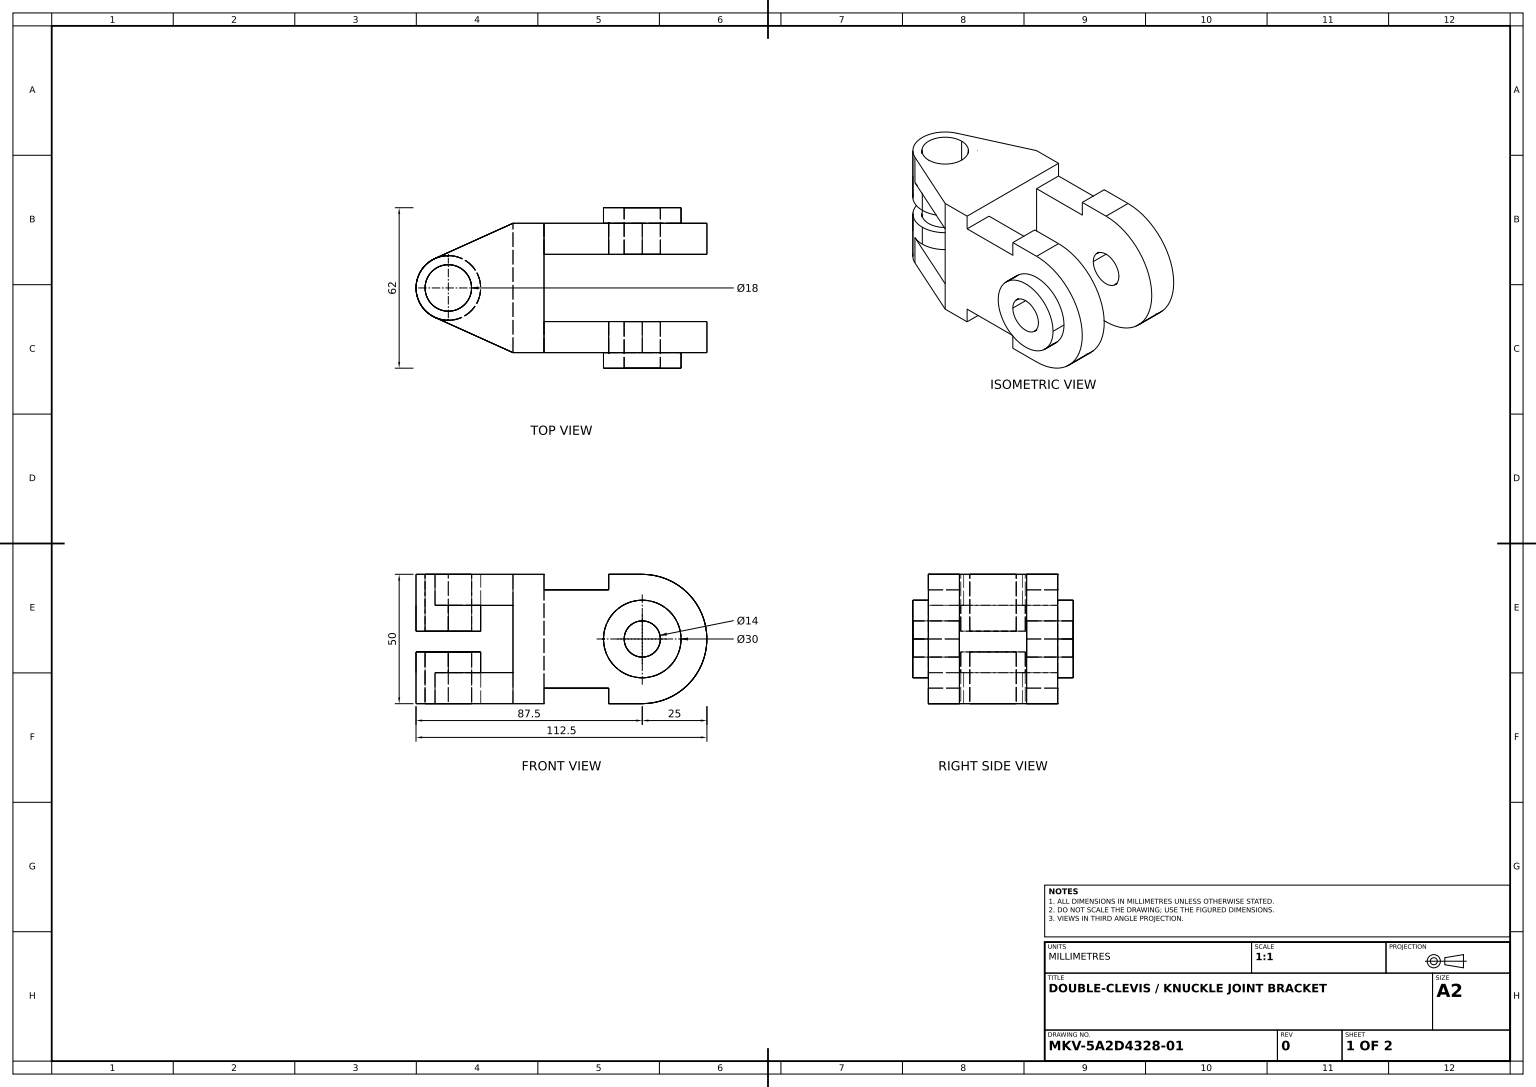
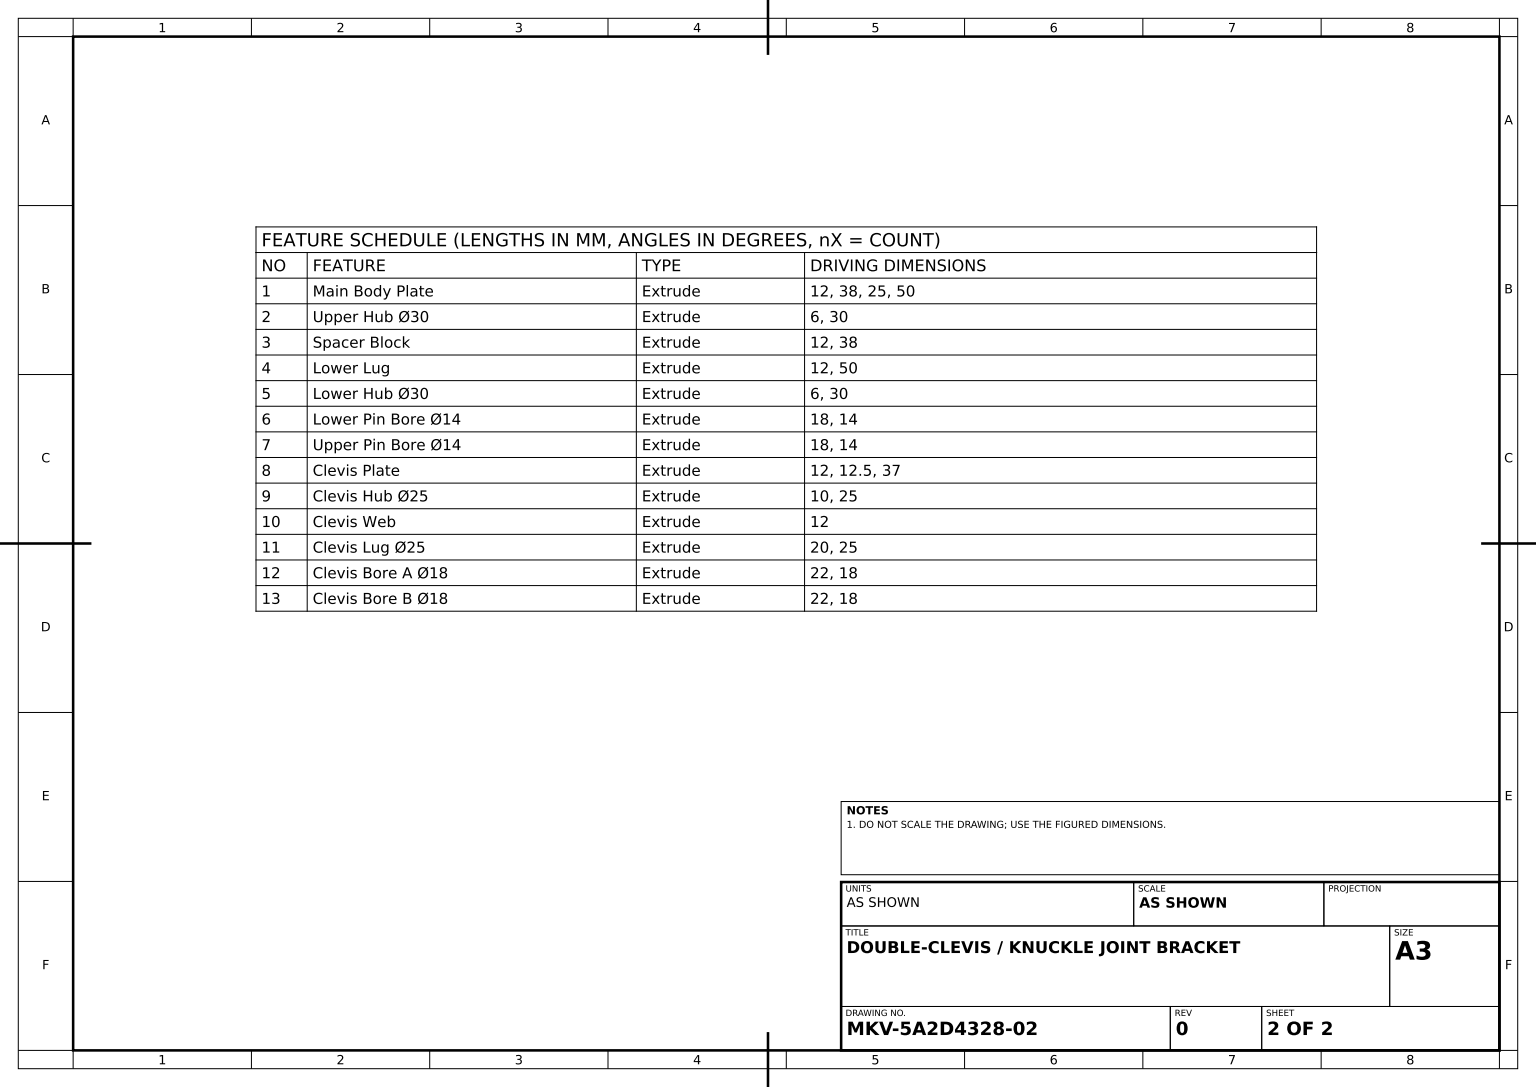
SolidWorks part; units mm, degrees
material "Plain Carbon Steel"
ref_plane "Front Plane" through (0, 0, 0) normal (0, 0, 1) x (1, 0, 0)
ref_plane "Top Plane" through (0, 0, 0) normal (0, 1, 0) x (1, 0, 0)
ref_plane "Right Plane" through (0, 0, 0) normal (1, 0, 0) x (0, 0, -1)
sketch "Main Body Profile Sketch" plane through (0, 0, 0) normal (0, 0, 1) x (1, 0, 0)
  line L0 (0, 0) -> (0, 50)
  line L1 (0, 50) -> (12, 50)
  line L2 (12, 50) -> (12, 44)
  line L3 (12, 44) -> (37, 44)
  line L4 (37, 44) -> (37, 50)
  line L5 (37, 50) -> (50, 50)
  line L7 (50, 0) -> (37, 0)
  line L8 (37, 0) -> (37, 6)
  line L9 (37, 6) -> (12, 6)
  line L10 (12, 6) -> (12, 0)
  line L11 (12, 0) -> (0, 0)
  arc A0 (50, 0) -> (50, 50) centre (50, 25) ccw
  dimension "D1" = 50
  dimension "D3" = 25
  dimension "D2" = 38
  dimension "D4" = 12
  dimension "D5" = 50
extrude "Main Body Plate" add sketch "Main Body Profile Sketch" along normal blind 12
sketch "Upper Hub Sketch" plane through (0, 0, 12) normal (0, 0, 1) x (1, 0, 0)
  circle A0 centre (50, 25) radius 15
  dimension "D1" = 30
  dimension "D2" = 30
extrude "Upper Hub Ø30" add sketch "Upper Hub Sketch" along normal blind 6
sketch "Spacer Block Sketch" plane through (0, 0, 0) normal (-1, 0, 0) x (0, 0, 1)
  line L0 (0, 50) -> (-38, 50)
  line L1 (-38, 50) -> (-38, 0)
  line L2 (-38, 0) -> (0, 0)
  line L3 (0, 0) -> (0, 50)
  line L4 (0, 50) -> (0, 0) construction
  dimension "D1" = 38
extrude "Spacer Block" add sketch "Spacer Block Sketch" against normal blind 12
sketch "Lower Lug Sketch" plane through (0, 0, -38) normal (0, 0, -1) x (-1, 0, 0)
  line L0 (0, 50) -> (0, 0) construction
  line L1 (-12, 44) -> (-37, 44)
  line L2 (-37, 44) -> (-37, 50)
  line L3 (-37, 50) -> (-50, 50)
  line L4 (-50, 50) -> (-37, 50) construction
  line L6 (-37, 0) -> (-50, 0) construction
  line L7 (-50, 0) -> (-37, 0)
  line L8 (-37, 0) -> (-37, 6)
  line L9 (-37, 6) -> (-12, 6)
  line L10 (-12, 6) -> (-12, 44)
  arc A1 (-50, 50) -> (-50, 0) centre (-50, 25) ccw
  dimension "D1" = 50
extrude "Lower Lug" add sketch "Lower Lug Sketch" against normal blind 12
sketch "Lower Hub Sketch" plane through (0, 0, -38) normal (0, 0, -1) x (-1, 0, 0)
  circle A0 centre (-50, 25) radius 15
  dimension "D1" = 30
  dimension "D2" = 30
extrude "Lower Hub Ø30" add sketch "Lower Hub Sketch" along normal blind 6
sketch "Lower Pin Bore Sketch" plane through (0, 0, -44) normal (0, 0, -1) x (-1, 0, 0)
  circle A0 centre (-50, 25) radius 7
  dimension "D1" = 14
  dimension "D2" = 14
extrude "Lower Pin Bore Ø14" cut sketch "Lower Pin Bore Sketch" against normal blind 18
sketch "Upper Pin Bore Sketch" plane through (0, 0, 18) normal (0, 0, 1) x (1, 0, 0)
  circle A0 centre (50, 25) radius 7
  dimension "D1" = 14
  dimension "D2" = 14
extrude "Upper Pin Bore Ø14" cut sketch "Upper Pin Bore Sketch" against normal blind 18
sketch "Clevis Plate Sketch" plane through (0, 50, 0) normal (0, 1, 0) x (1, 0, 0)
  line L0 (12, -12) -> (12, 38) construction
  line L2 (0, 38) -> (-30.143, 24.393)
  line L3 (0, -12) -> (-30.143, 1.607)
  line L7 (12, -12) -> (12, 38)
  line L8 (12, 38) -> (0, 38)
  line L9 (0, 38) -> (0, -12)
  line L10 (0, -12) -> (12, -12)
  line L13 (0, 38) -> (0, -12)
  arc A0 (-30.143, 24.393) -> (-30.143, 1.607) centre (-25, 13) ccw
  dimension "D1" = 25
  dimension "D3" = 12.5
  dimension "D2" = 0
  dimension "D4" = 37
extrude "Clevis Plate" add sketch "Clevis Plate Sketch" against normal blind 12
sketch "Clevis Hub Sketch" plane through (0, 38, 0) normal (0, -1, 0) x (1, 0, 0)
  circle A0 centre (-25, -13) radius 12.5
  dimension "D1" = 25
  dimension "D2" = 25
extrude "Clevis Hub Ø25" add sketch "Clevis Hub Sketch" along normal blind 10
sketch "Clevis Web Sketch" plane through (0, 0, 0) normal (0, -1, 0) x (1, 0, 0)
  line L0 (0, 12) -> (-30.143, -1.607)
  line L1 (0, -38) -> (-30.143, -24.393)
  line L2 (0, 12) -> (0, -38)
  circle A0 centre (-25, -13) radius 12.5
  line M1 (0, 12) -> (0, -38)
  dimension "D1" = 25
extrude "Clevis Web" add sketch "Clevis Web Sketch" against normal blind 12 contours A0 L1 L0 M1
sketch "Clevis Lug Sketch" plane through (0, 0, 0) normal (0, -1, 0) x (1, 0, 0)
  circle A0 centre (-25, -13) radius 12.5
  dimension "D1" = 25
  dimension "D2" = 25
extrude "Clevis Lug Ø25" add sketch "Clevis Lug Sketch" against normal blind 20
sketch "Clevis Bore A Sketch" plane through (0, 50, 0) normal (0, 1, 0) x (1, 0, 0)
  circle A0 centre (-25, 13) radius 9
  dimension "D1" = 18
  dimension "D2" = 18
extrude "Clevis Bore A Ø18" cut sketch "Clevis Bore A Sketch" against normal blind 22
sketch "Clevis Bore B Sketch" plane through (0, 0, 0) normal (0, -1, 0) x (1, 0, 0)
  circle A0 centre (-25, -13) radius 9
  dimension "D1" = 18
  dimension "D2" = 18
extrude "Clevis Bore B Ø18" cut sketch "Clevis Bore B Sketch" against normal blind 22
